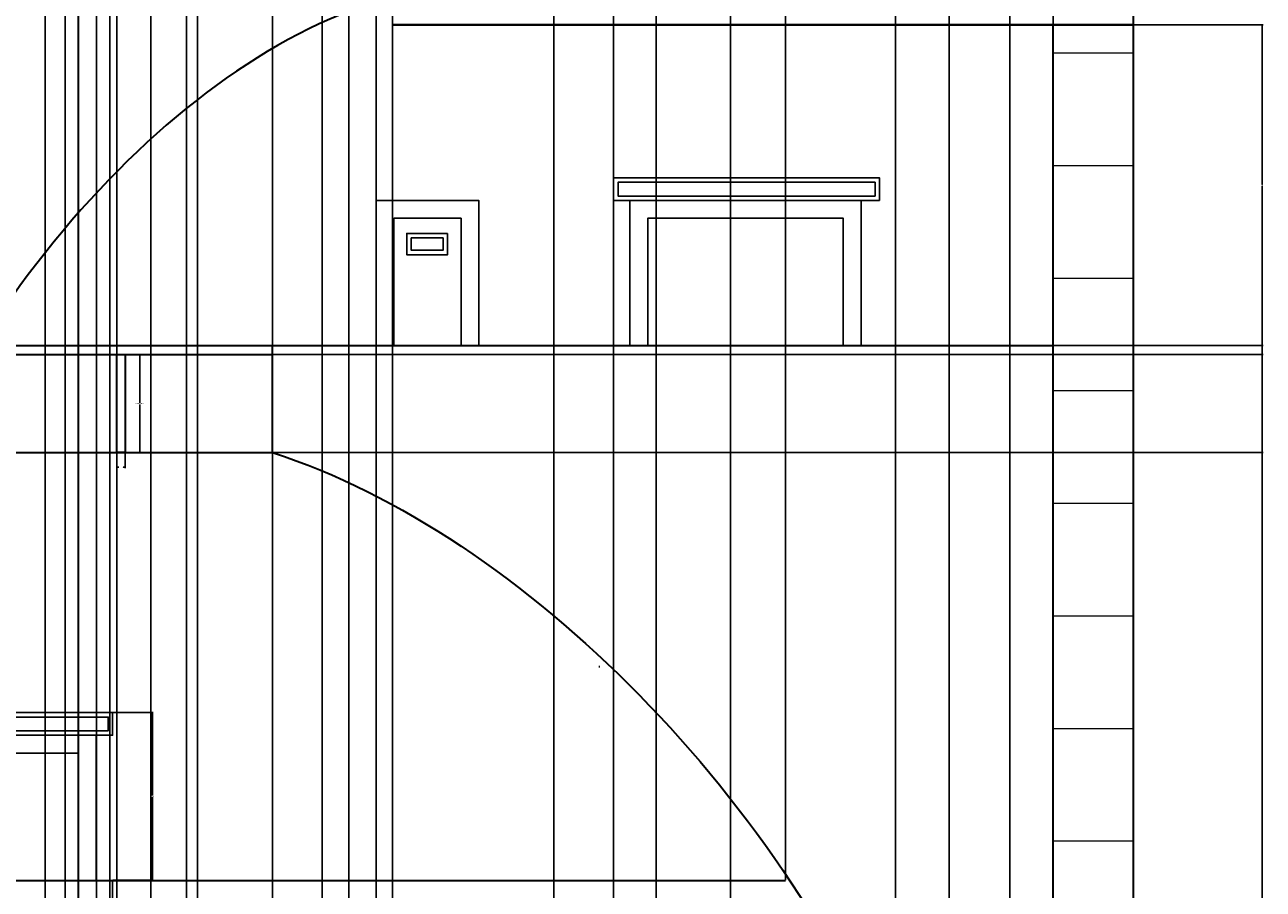
# Model space of a CAD drawing. Units: inches. Extents: x -19 to 408, y -26 to 603.
# Tile 6 of 7: x 130 to 408, y 289 to 483. Entities that reach past the tile are written whole.
import ezdxf

# ---------------------------------------------------------------- set-up
doc = ezdxf.new("R2010")
doc.units = ezdxf.units.IN
doc.header["$MEASUREMENT"] = 0
for name, color, linetype, lineweight in [('A-ANNO-DIMS', 2, 'Continuous', 18), ('A-DOOR', 3, 'Continuous', 25), ('A-ELEV', 7, 'Continuous', 35), ('A-GLAZ', 4, 'Continuous', 25), ('A-WALL-PATT', 8, 'Continuous', 13)]:
    doc.layers.add(name, color=color, linetype=linetype, lineweight=lineweight)
doc.styles.get("Standard").update_dxf_attribs({"font": 'arial.ttf'})
doc.dimstyles.get("Standard").update_dxf_attribs({"dimtxt": 0.18, "dimasz": 0.18, "dimexe": 0.18, "dimexo": 0.0625, "dimgap": 0.09, "dimtad": 0, "dimtih": 1, "dimtoh": 1, "dimdec": 4, "dimzin": 0, "dimdsep": 46, "dimtxsty": 'Standard', "dimcen": 0.09, "dimadec": 0, "dimazin": 0, "dimtfac": 1, "dimtdec": 4, "dimtofl": 0, "dimtmove": 0, "dimatfit": 3, "dimfxl": 1, "dimtolj": 1, "dimtzin": 0, "dimarcsym": 0})

# ---------------------------------------------------------------- blocks, each defined once
blk = doc.blocks.new('WIN-1200')
for points in [[(0, 32.56), (59.66, 32.56), (59.66, 37.64), (0, 37.64)], [(1, 33.56), (58.66, 33.56), (58.66, 36.64), (1, 36.64)]]:
    blk.add_lwpolyline(points, close=True)
for points in [[(4.17, 0), (4.17, 32.56), (55.99, 32.56), (55.99, 0)], [(8.17, 0), (8.17, 28.56), (51.99, 28.56), (51.99, 0)]]:
    blk.add_lwpolyline(points)
blk = doc.blocks.new('DOOR-600')
for points in [[(0, 0), (0, 32.56), (23.06, 32.56), (23.06, 0)], [(4, 0), (4, 28.56), (19.06, 28.56), (19.06, 0)]]:
    blk.add_lwpolyline(points)
for points in [[(7.03, 25.16), (16.18, 25.16), (16.18, 20.4), (7.03, 20.4)], [(8.03, 24.16), (15.18, 24.16), (15.18, 21.4), (8.03, 21.4)]]:
    blk.add_lwpolyline(points, close=True)
blk = doc.blocks.new('RAIL-POST')
blk.add_lwpolyline([(0, 22), (1.83, 22), (1.83, 0), (0, 0)], close=True)
blk = doc.blocks.new('*D4')
at = {"layer": 'A-ANNO-DIMS', "color": 0, "lineweight": -2, "transparency": 16777216}
for p, q in [((89.99, 291.08), (89.99, 282.02)), ((149.65, 291.08), (149.65, 282.02)), ((90.17, 282.2), (118.7, 282.2)), ((149.47, 282.2), (120.94, 282.2))]:
    blk.add_line(p, q, dxfattribs=at)
at = {"layer": 'A-ANNO-DIMS', "color": 0, "transparency": 16777216}
for points in [[(90.17, 282.23), (90.17, 282.17), (89.99, 282.2)], [(149.47, 282.23), (149.47, 282.17), (149.65, 282.2)]]:
    blk.add_solid(points, dxfattribs=at)
at = {"layer": 'Defpoints', "color": 0, "transparency": 16777216}
for p in [(89.99, 291.15), (149.65, 291.15), (149.65, 282.2)]:
    blk.add_point(p, dxfattribs=at)
at = {"layer": 'A-ANNO-DIMS', "color": 0, "transparency": 16777216, "insert": (119.82, 282.2), "char_height": 0.18, "attachment_point": 5}
blk.add_mtext('\\A1;WINDOW 60 TYP.', dxfattribs=at)
blk = doc.blocks.new('*D5')
at = {"layer": 'A-ANNO-DIMS', "color": 0, "lineweight": -2, "transparency": 16777216}
for p, q in [((149.71, 328.79), (158.77, 328.79)), ((158.59, 328.61), (158.59, 310.15)), ((158.59, 291.33), (158.59, 309.79)), ((149.71, 291.15), (158.77, 291.15))]:
    blk.add_line(p, q, dxfattribs=at)
at = {"layer": 'A-ANNO-DIMS', "color": 0, "transparency": 16777216}
for points in [[(158.56, 328.61), (158.62, 328.61), (158.59, 328.79)], [(158.56, 291.33), (158.62, 291.33), (158.59, 291.15)]]:
    blk.add_solid(points, dxfattribs=at)
at = {"layer": 'Defpoints', "color": 0, "transparency": 16777216}
for p in [(149.65, 328.79), (158.59, 328.79), (149.65, 291.15)]:
    blk.add_point(p, dxfattribs=at)
at = {"layer": 'A-ANNO-DIMS', "color": 0, "transparency": 16777216, "insert": (158.59, 309.97), "char_height": 0.18, "attachment_point": 5}
blk.add_mtext('\\A1;38 TYP.', dxfattribs=at)
blk = doc.blocks.new('*D8')
at = {"layer": 'A-ANNO-DIMS', "color": 0, "lineweight": -2, "transparency": 16777216}
for p, q in [((152.51, 409.15), (155.92, 409.15)), ((155.74, 408.97), (155.74, 398.33)), ((155.74, 387.33), (155.74, 397.96)), ((152.51, 387.15), (155.92, 387.15))]:
    blk.add_line(p, q, dxfattribs=at)
at = {"layer": 'A-ANNO-DIMS', "color": 0, "transparency": 16777216}
for points in [[(155.71, 408.97), (155.77, 408.97), (155.74, 409.15)], [(155.71, 387.33), (155.77, 387.33), (155.74, 387.15)]]:
    blk.add_solid(points, dxfattribs=at)
at = {"layer": 'Defpoints', "color": 0, "transparency": 16777216}
for p in [(152.44, 409.15), (155.74, 409.15), (152.44, 387.15)]:
    blk.add_point(p, dxfattribs=at)
at = {"layer": 'A-ANNO-DIMS', "color": 0, "transparency": 16777216, "insert": (155.74, 398.15), "char_height": 0.18, "attachment_point": 5}
blk.add_mtext('\\A1;RAIL POST 22 TYP.', dxfattribs=at)
blk = doc.blocks.new('*D9')
at = {"layer": 'A-ANNO-DIMS', "color": 0, "lineweight": -2, "transparency": 16777216}
for p, q in [((150.62, 387.08), (150.62, 383.67)), ((152.44, 387.08), (152.44, 383.67)), ((150.8, 383.85), (151.07, 383.85)), ((152.26, 383.85), (151.99, 383.85))]:
    blk.add_line(p, q, dxfattribs=at)
at = {"layer": 'A-ANNO-DIMS', "color": 0, "transparency": 16777216}
for points in [[(150.8, 383.88), (150.8, 383.82), (150.62, 383.85)], [(152.26, 383.88), (152.26, 383.82), (152.44, 383.85)]]:
    blk.add_solid(points, dxfattribs=at)
at = {"layer": 'Defpoints', "color": 0, "transparency": 16777216}
for p in [(150.62, 387.15), (152.44, 387.15), (152.44, 383.85)]:
    blk.add_point(p, dxfattribs=at)
at = {"layer": 'A-ANNO-DIMS', "color": 0, "transparency": 16777216, "insert": (151.53, 383.85), "char_height": 0.18, "attachment_point": 5}
blk.add_mtext('\\A1;2 TYP.', dxfattribs=at)
blk = doc.blocks.new('*D20')
at = {"layer": 'A-ANNO-DIMS', "color": 0, "lineweight": -2, "transparency": 16777216}
for p, q in [((185.46, 411.15), (-18.88, 411.15)), ((-18.7, 410.97), (-18.7, 351.33)), ((-18.7, 291.33), (-18.7, 350.97)), ((84.02, 291.15), (-18.88, 291.15))]:
    blk.add_line(p, q, dxfattribs=at)
at = {"layer": 'A-ANNO-DIMS', "color": 0, "transparency": 16777216}
for points in [[(-18.73, 410.97), (-18.67, 410.97), (-18.7, 411.15)], [(-18.73, 291.33), (-18.67, 291.33), (-18.7, 291.15)]]:
    blk.add_solid(points, dxfattribs=at)
at = {"layer": 'Defpoints', "color": 0, "transparency": 16777216}
for p in [(-18.7, 411.15), (185.52, 411.15), (84.08, 291.15)]:
    blk.add_point(p, dxfattribs=at)
at = {"layer": 'A-ANNO-DIMS', "color": 0, "transparency": 16777216, "insert": (-18.7, 351.15), "char_height": 0.18, "attachment_point": 5}
blk.add_mtext('\\A1;120', dxfattribs=at)
blk = doc.blocks.new('*D21')
at = {"layer": 'A-ANNO-DIMS', "color": 0, "lineweight": -2, "transparency": 16777216}
for p, q in [((212.37, 551.1), (-18.88, 551.1)), ((-18.7, 550.92), (-18.7, 481.31)), ((-18.7, 411.33), (-18.7, 480.94)), ((185.46, 411.15), (-18.88, 411.15))]:
    blk.add_line(p, q, dxfattribs=at)
at = {"layer": 'A-ANNO-DIMS', "color": 0, "transparency": 16777216}
for points in [[(-18.73, 550.92), (-18.67, 550.92), (-18.7, 551.1)], [(-18.73, 411.33), (-18.67, 411.33), (-18.7, 411.15)]]:
    blk.add_solid(points, dxfattribs=at)
at = {"layer": 'Defpoints', "color": 0, "transparency": 16777216}
for p in [(-18.7, 551.1), (212.43, 551.1), (185.52, 411.15)]:
    blk.add_point(p, dxfattribs=at)
at = {"layer": 'A-ANNO-DIMS', "color": 0, "transparency": 16777216, "insert": (-18.7, 481.13), "char_height": 0.18, "attachment_point": 5}
blk.add_mtext('\\A1;139.96', dxfattribs=at)
blk = doc.blocks.new('*D23')
at = {"layer": 'A-ANNO-DIMS', "color": 0, "lineweight": -2, "transparency": 16777216}
for p, q in [((360.63, 411.15), (407.65, 411.15)), ((407.47, 410.97), (407.47, 267.33)), ((407.47, 123.33), (407.47, 266.97)), ((360.63, 123.15), (407.65, 123.15))]:
    blk.add_line(p, q, dxfattribs=at)
at = {"layer": 'A-ANNO-DIMS', "color": 0, "transparency": 16777216}
for points in [[(407.44, 410.97), (407.5, 410.97), (407.47, 411.15)], [(407.44, 123.33), (407.5, 123.33), (407.47, 123.15)]]:
    blk.add_solid(points, dxfattribs=at)
at = {"layer": 'Defpoints', "color": 0, "transparency": 16777216}
for p in [(360.57, 411.15), (407.47, 411.15), (360.57, 123.15)]:
    blk.add_point(p, dxfattribs=at)
at = {"layer": 'A-ANNO-DIMS', "color": 0, "transparency": 16777216, "insert": (407.47, 267.15), "char_height": 0.18, "attachment_point": 5}
blk.add_mtext('\\A1;288', dxfattribs=at)
blk = doc.blocks.new('*D24')
at = {"layer": 'A-ANNO-DIMS', "color": 0, "lineweight": -2, "transparency": 16777216}
for p, q in [((378.63, 483.15), (407.65, 483.15)), ((407.47, 482.97), (407.47, 447.33)), ((407.47, 411.33), (407.47, 446.97)), ((360.63, 411.15), (407.65, 411.15))]:
    blk.add_line(p, q, dxfattribs=at)
at = {"layer": 'A-ANNO-DIMS', "color": 0, "transparency": 16777216}
for points in [[(407.44, 482.97), (407.5, 482.97), (407.47, 483.15)], [(407.44, 411.33), (407.5, 411.33), (407.47, 411.15)]]:
    blk.add_solid(points, dxfattribs=at)
at = {"layer": 'Defpoints', "color": 0, "transparency": 16777216}
for p in [(378.57, 483.15), (407.47, 483.15), (360.57, 411.15)]:
    blk.add_point(p, dxfattribs=at)
at = {"layer": 'A-ANNO-DIMS', "color": 0, "transparency": 16777216, "insert": (407.47, 447.15), "char_height": 0.18, "attachment_point": 5}
blk.add_mtext('\\A1;72', dxfattribs=at)
blk = doc.blocks.new('*D27')
at = {"layer": 'A-ANNO-DIMS', "color": 0, "lineweight": -2, "transparency": 16777216}
for p, q in [((288.17, 123.21), (288.17, 602.9)), ((288.35, 602.72), (324.05, 602.72)), ((360.39, 602.72), (324.69, 602.72)), ((360.57, 123.21), (360.57, 602.9))]:
    blk.add_line(p, q, dxfattribs=at)
at = {"layer": 'A-ANNO-DIMS', "color": 0, "transparency": 16777216}
for points in [[(288.35, 602.75), (288.35, 602.69), (288.17, 602.72)], [(360.39, 602.75), (360.39, 602.69), (360.57, 602.72)]]:
    blk.add_solid(points, dxfattribs=at)
at = {"layer": 'Defpoints', "color": 0, "transparency": 16777216}
for p in [(360.57, 602.72), (288.17, 123.15), (360.57, 123.15)]:
    blk.add_point(p, dxfattribs=at)
at = {"layer": 'A-ANNO-DIMS', "color": 0, "transparency": 16777216, "insert": (324.37, 602.72), "char_height": 0.18, "attachment_point": 5}
blk.add_mtext('\\A1;72.4', dxfattribs=at)
blk = doc.blocks.new('*D29')
at = {"layer": 'A-ANNO-DIMS', "color": 0, "lineweight": -2, "transparency": 16777216}
for p, q in [((300.56, 291.21), (300.56, 602.9)), ((300.74, 602.72), (330.19, 602.72)), ((360.39, 602.72), (330.94, 602.72)), ((360.57, 300.05), (360.57, 602.9))]:
    blk.add_line(p, q, dxfattribs=at)
at = {"layer": 'A-ANNO-DIMS', "color": 0, "transparency": 16777216}
for points in [[(300.74, 602.75), (300.74, 602.69), (300.56, 602.72)], [(360.39, 602.75), (360.39, 602.69), (360.57, 602.72)]]:
    blk.add_solid(points, dxfattribs=at)
at = {"layer": 'Defpoints', "color": 0, "transparency": 16777216}
for p in [(360.57, 602.72), (360.57, 299.99), (300.56, 291.15)]:
    blk.add_point(p, dxfattribs=at)
at = {"layer": 'A-ANNO-DIMS', "color": 0, "transparency": 16777216, "insert": (330.56, 602.72), "char_height": 0.18, "attachment_point": 5}
blk.add_mtext('\\A1;60.01', dxfattribs=at)
blk = doc.blocks.new('*D30')
at = {"layer": 'A-ANNO-DIMS', "color": 0, "lineweight": -2, "transparency": 16777216}
for p, q in [((360.57, 411.08), (360.57, -25.93)), ((185.52, 387.08), (185.52, -25.93)), ((185.7, -25.75), (272.59, -25.75)), ((360.39, -25.75), (273.5, -25.75))]:
    blk.add_line(p, q, dxfattribs=at)
at = {"layer": 'A-ANNO-DIMS', "color": 0, "transparency": 16777216}
for points in [[(185.7, -25.72), (185.7, -25.78), (185.52, -25.75)], [(360.39, -25.72), (360.39, -25.78), (360.57, -25.75)]]:
    blk.add_solid(points, dxfattribs=at)
at = {"layer": 'Defpoints', "color": 0, "transparency": 16777216}
for p in [(360.57, 411.15), (185.52, 387.15), (360.57, -25.75)]:
    blk.add_point(p, dxfattribs=at)
at = {"layer": 'A-ANNO-DIMS', "color": 0, "transparency": 16777216, "insert": (273.05, -25.75), "char_height": 0.18, "attachment_point": 5}
blk.add_mtext('\\A1;175.05', dxfattribs=at)
blk = doc.blocks.new('*D36')
at = {"layer": 'A-ANNO-DIMS', "color": 0, "lineweight": -2, "transparency": 16777216}
for p, q in [((52.15, 203.77), (52.15, 602.9)), ((52.33, 602.72), (96.69, 602.72)), ((141.84, 602.72), (97.48, 602.72)), ((142.02, 171.21), (142.02, 602.9))]:
    blk.add_line(p, q, dxfattribs=at)
at = {"layer": 'A-ANNO-DIMS', "color": 0, "transparency": 16777216}
for points in [[(52.33, 602.75), (52.33, 602.69), (52.15, 602.72)], [(141.84, 602.75), (141.84, 602.69), (142.02, 602.72)]]:
    blk.add_solid(points, dxfattribs=at)
at = {"layer": 'Defpoints', "color": 0, "transparency": 16777216}
for p in [(142.02, 602.72), (52.15, 203.7), (142.02, 171.15)]:
    blk.add_point(p, dxfattribs=at)
at = {"layer": 'A-ANNO-DIMS', "color": 0, "transparency": 16777216, "insert": (97.09, 602.72), "char_height": 0.18, "attachment_point": 5}
blk.add_mtext('\\A1;89.87', dxfattribs=at)
blk = doc.blocks.new('*D37')
at = {"layer": 'A-ANNO-DIMS', "color": 0, "lineweight": -2, "transparency": 16777216}
for p, q in [((142.02, 171.21), (142.02, 602.9)), ((142.2, 602.72), (174.97, 602.72)), ((208.53, 602.72), (175.76, 602.72)), ((208.71, 171.21), (208.71, 602.9))]:
    blk.add_line(p, q, dxfattribs=at)
at = {"layer": 'A-ANNO-DIMS', "color": 0, "transparency": 16777216}
for points in [[(142.2, 602.75), (142.2, 602.69), (142.02, 602.72)], [(208.53, 602.75), (208.53, 602.69), (208.71, 602.72)]]:
    blk.add_solid(points, dxfattribs=at)
at = {"layer": 'Defpoints', "color": 0, "transparency": 16777216}
for p in [(208.71, 602.72), (142.02, 171.15), (208.71, 171.15)]:
    blk.add_point(p, dxfattribs=at)
at = {"layer": 'A-ANNO-DIMS', "color": 0, "transparency": 16777216, "insert": (175.37, 602.72), "char_height": 0.18, "attachment_point": 5}
blk.add_mtext('\\A1;66.69', dxfattribs=at)
blk = doc.blocks.new('*D38')
at = {"layer": 'A-ANNO-DIMS', "color": 0, "lineweight": -2, "transparency": 16777216}
for p, q in [((208.71, 171.21), (208.71, 602.9)), ((208.89, 602.72), (234.95, 602.72)), ((261.81, 602.72), (235.74, 602.72)), ((261.99, 203.77), (261.99, 602.9))]:
    blk.add_line(p, q, dxfattribs=at)
at = {"layer": 'A-ANNO-DIMS', "color": 0, "transparency": 16777216}
for points in [[(208.89, 602.75), (208.89, 602.69), (208.71, 602.72)], [(261.81, 602.75), (261.81, 602.69), (261.99, 602.72)]]:
    blk.add_solid(points, dxfattribs=at)
at = {"layer": 'Defpoints', "color": 0, "transparency": 16777216}
for p in [(261.99, 602.72), (261.99, 203.7), (208.71, 171.15)]:
    blk.add_point(p, dxfattribs=at)
at = {"layer": 'A-ANNO-DIMS', "color": 0, "transparency": 16777216, "insert": (235.35, 602.72), "char_height": 0.18, "attachment_point": 5}
blk.add_mtext('\\A1;53.28', dxfattribs=at)
blk = doc.blocks.new('*D45')
at = {"layer": 'A-ANNO-DIMS', "color": 0, "lineweight": -2, "transparency": 16777216}
for p, q in [((36.57, 219.21), (36.57, 602.9)), ((36.75, 602.72), (85.2, 602.72)), ((134.3, 602.72), (85.85, 602.72)), ((134.48, 220.21), (134.48, 602.9))]:
    blk.add_line(p, q, dxfattribs=at)
at = {"layer": 'A-ANNO-DIMS', "color": 0, "transparency": 16777216}
for points in [[(36.75, 602.75), (36.75, 602.69), (36.57, 602.72)], [(134.3, 602.75), (134.3, 602.69), (134.48, 602.72)]]:
    blk.add_solid(points, dxfattribs=at)
at = {"layer": 'Defpoints', "color": 0, "transparency": 16777216}
for p in [(134.48, 602.72), (134.48, 220.15), (36.57, 219.15)]:
    blk.add_point(p, dxfattribs=at)
at = {"layer": 'A-ANNO-DIMS', "color": 0, "transparency": 16777216, "insert": (85.52, 602.72), "char_height": 0.18, "attachment_point": 5}
blk.add_mtext('\\A1;97.9', dxfattribs=at)
blk = doc.blocks.new('*D46')
at = {"layer": 'A-ANNO-DIMS', "color": 0, "lineweight": -2, "transparency": 16777216}
for p, q in [((337.23, 171.21), (337.23, 602.9)), ((337.41, 602.72), (348.43, 602.72)), ((360.39, 602.72), (349.36, 602.72)), ((360.57, 173.74), (360.57, 602.9))]:
    blk.add_line(p, q, dxfattribs=at)
at = {"layer": 'A-ANNO-DIMS', "color": 0, "transparency": 16777216}
for points in [[(337.41, 602.75), (337.41, 602.69), (337.23, 602.72)], [(360.39, 602.75), (360.39, 602.69), (360.57, 602.72)]]:
    blk.add_solid(points, dxfattribs=at)
at = {"layer": 'Defpoints', "color": 0, "transparency": 16777216}
for p in [(360.57, 602.72), (360.57, 173.67), (337.23, 171.15)]:
    blk.add_point(p, dxfattribs=at)
at = {"layer": 'A-ANNO-DIMS', "color": 0, "transparency": 16777216, "insert": (348.9, 602.72), "char_height": 0.18, "attachment_point": 5}
blk.add_mtext('\\A1;23.345', dxfattribs=at)
blk = doc.blocks.new('*D55')
at = {"layer": 'A-ANNO-DIMS', "color": 0, "lineweight": -2, "transparency": 16777216}
for p, q in [((146.02, 199.77), (146.02, 602.9)), ((146.2, 602.72), (147.14, 602.72)), ((148.87, 602.72), (147.93, 602.72)), ((149.05, 196.37), (149.05, 602.9))]:
    blk.add_line(p, q, dxfattribs=at)
at = {"layer": 'A-ANNO-DIMS', "color": 0, "transparency": 16777216}
for points in [[(146.2, 602.75), (146.2, 602.69), (146.02, 602.72)], [(148.87, 602.75), (148.87, 602.69), (149.05, 602.72)]]:
    blk.add_solid(points, dxfattribs=at)
at = {"layer": 'Defpoints', "color": 0, "transparency": 16777216}
for p in [(149.05, 602.72), (146.02, 199.7), (149.05, 196.31)]:
    blk.add_point(p, dxfattribs=at)
at = {"layer": 'A-ANNO-DIMS', "color": 0, "transparency": 16777216, "insert": (147.54, 602.72), "char_height": 0.18, "attachment_point": 5}
blk.add_mtext('\\A1;3.029', dxfattribs=at)
blk = doc.blocks.new('*D56')
at = {"layer": 'A-ANNO-DIMS', "color": 0, "lineweight": -2, "transparency": 16777216}
for p, q in [((149.05, 196.37), (149.05, 602.9)), ((149.23, 602.72), (153.3, 602.72)), ((158.02, 602.72), (153.95, 602.72)), ((158.2, 196.37), (158.2, 602.9))]:
    blk.add_line(p, q, dxfattribs=at)
at = {"layer": 'A-ANNO-DIMS', "color": 0, "transparency": 16777216}
for points in [[(149.23, 602.75), (149.23, 602.69), (149.05, 602.72)], [(158.02, 602.75), (158.02, 602.69), (158.2, 602.72)]]:
    blk.add_solid(points, dxfattribs=at)
at = {"layer": 'Defpoints', "color": 0, "transparency": 16777216}
for p in [(158.2, 602.72), (149.05, 196.31), (158.2, 196.31)]:
    blk.add_point(p, dxfattribs=at)
at = {"layer": 'A-ANNO-DIMS', "color": 0, "transparency": 16777216, "insert": (153.63, 602.72), "char_height": 0.18, "attachment_point": 5}
blk.add_mtext('\\A1;9.15', dxfattribs=at)
blk = doc.blocks.new('*D70')
at = {"layer": 'A-ANNO-DIMS', "color": 0, "lineweight": -2, "transparency": 16777216}
for p, q in [((150.62, 387.08), (150.62, -25.93)), ((185.52, 387.08), (185.52, -25.93)), ((150.8, -25.75), (167.6, -25.75)), ((185.34, -25.75), (168.53, -25.75))]:
    blk.add_line(p, q, dxfattribs=at)
at = {"layer": 'A-ANNO-DIMS', "color": 0, "transparency": 16777216}
for points in [[(150.8, -25.72), (150.8, -25.78), (150.62, -25.75)], [(185.34, -25.72), (185.34, -25.78), (185.52, -25.75)]]:
    blk.add_solid(points, dxfattribs=at)
at = {"layer": 'Defpoints', "color": 0, "transparency": 16777216}
for p in [(150.62, 387.15), (185.52, 387.15), (185.52, -25.75)]:
    blk.add_point(p, dxfattribs=at)
at = {"layer": 'A-ANNO-DIMS', "color": 0, "transparency": 16777216, "insert": (168.07, -25.75), "char_height": 0.18, "attachment_point": 5}
blk.add_mtext('\\A1;34.906', dxfattribs=at)
blk = doc.blocks.new('*D71')
at = {"layer": 'A-ANNO-DIMS', "color": 0, "lineweight": -2, "transparency": 16777216}
for p, q in [((185.58, 409.15), (407.65, 409.15)), ((407.47, 408.97), (407.47, 398.33)), ((407.47, 387.33), (407.47, 397.97)), ((185.58, 387.15), (407.65, 387.15))]:
    blk.add_line(p, q, dxfattribs=at)
at = {"layer": 'A-ANNO-DIMS', "color": 0, "transparency": 16777216}
for points in [[(407.44, 408.97), (407.5, 408.97), (407.47, 409.15)], [(407.44, 387.33), (407.5, 387.33), (407.47, 387.15)]]:
    blk.add_solid(points, dxfattribs=at)
at = {"layer": 'Defpoints', "color": 0, "transparency": 16777216}
for p in [(185.52, 409.15), (407.47, 409.15), (185.52, 387.15)]:
    blk.add_point(p, dxfattribs=at)
at = {"layer": 'A-ANNO-DIMS', "color": 0, "transparency": 16777216, "insert": (407.47, 398.15), "char_height": 0.18, "attachment_point": 5}
blk.add_mtext('\\A1;22', dxfattribs=at)
blk = doc.blocks.new('*D72')
at = {"layer": 'A-ANNO-DIMS', "color": 0, "lineweight": -2, "transparency": 16777216}
for p, q in [((185.58, 411.15), (407.65, 411.15)), ((185.58, 409.15), (407.65, 409.15)), ((407.47, 410.97), (407.47, 410.33)), ((407.47, 409.33), (407.47, 409.97))]:
    blk.add_line(p, q, dxfattribs=at)
at = {"layer": 'A-ANNO-DIMS', "color": 0, "transparency": 16777216}
for points in [[(407.44, 410.97), (407.5, 410.97), (407.47, 411.15)], [(407.44, 409.33), (407.5, 409.33), (407.47, 409.15)]]:
    blk.add_solid(points, dxfattribs=at)
at = {"layer": 'Defpoints', "color": 0, "transparency": 16777216}
for p in [(185.52, 411.15), (407.47, 411.15), (185.52, 409.15)]:
    blk.add_point(p, dxfattribs=at)
at = {"layer": 'A-ANNO-DIMS', "color": 0, "transparency": 16777216, "insert": (407.47, 410.15), "char_height": 0.18, "attachment_point": 5}
blk.add_mtext('\\A1;2', dxfattribs=at)
blk = doc.blocks.new('*D73')
at = {"layer": 'A-ANNO-DIMS', "color": 0, "lineweight": -2, "transparency": 16777216}
for p, q in [((185.52, 411.08), (185.52, -25.93)), ((208.71, 411.08), (208.71, -25.93)), ((185.7, -25.75), (196.72, -25.75)), ((208.53, -25.75), (197.51, -25.75))]:
    blk.add_line(p, q, dxfattribs=at)
at = {"layer": 'A-ANNO-DIMS', "color": 0, "transparency": 16777216}
for points in [[(185.7, -25.72), (185.7, -25.78), (185.52, -25.75)], [(208.53, -25.72), (208.53, -25.78), (208.71, -25.75)]]:
    blk.add_solid(points, dxfattribs=at)
at = {"layer": 'Defpoints', "color": 0, "transparency": 16777216}
for p in [(185.52, 411.15), (208.71, 411.15), (208.71, -25.75)]:
    blk.add_point(p, dxfattribs=at)
at = {"layer": 'A-ANNO-DIMS', "color": 0, "transparency": 16777216, "insert": (197.12, -25.75), "char_height": 0.18, "attachment_point": 5}
blk.add_mtext('\\A1;23.19', dxfattribs=at)
blk = doc.blocks.new('*D74')
at = {"layer": 'A-ANNO-DIMS', "color": 0, "lineweight": -2, "transparency": 16777216}
for p, q in [((208.71, 411.21), (208.71, 602.9)), ((208.89, 602.72), (234.95, 602.72)), ((261.81, 602.72), (235.74, 602.72)), ((261.99, 443.77), (261.99, 602.9))]:
    blk.add_line(p, q, dxfattribs=at)
at = {"layer": 'A-ANNO-DIMS', "color": 0, "transparency": 16777216}
for points in [[(208.89, 602.75), (208.89, 602.69), (208.71, 602.72)], [(261.81, 602.75), (261.81, 602.69), (261.99, 602.72)]]:
    blk.add_solid(points, dxfattribs=at)
at = {"layer": 'Defpoints', "color": 0, "transparency": 16777216}
for p in [(261.99, 602.72), (261.99, 443.7), (208.71, 411.15)]:
    blk.add_point(p, dxfattribs=at)
at = {"layer": 'A-ANNO-DIMS', "color": 0, "transparency": 16777216, "insert": (235.35, 602.72), "char_height": 0.18, "attachment_point": 5}
blk.add_mtext('\\A1;53.28', dxfattribs=at)
blk = doc.blocks.new('*D75')
at = {"layer": 'A-ANNO-DIMS', "color": 0, "lineweight": -2, "transparency": 16777216}
for p, q in [((212.43, 507.08), (212.43, -25.93)), ((248.57, 507.08), (248.57, -25.93)), ((212.61, -25.75), (230.11, -25.75)), ((248.39, -25.75), (230.89, -25.75))]:
    blk.add_line(p, q, dxfattribs=at)
at = {"layer": 'A-ANNO-DIMS', "color": 0, "transparency": 16777216}
for points in [[(212.61, -25.72), (212.61, -25.78), (212.43, -25.75)], [(248.39, -25.72), (248.39, -25.78), (248.57, -25.75)]]:
    blk.add_solid(points, dxfattribs=at)
at = {"layer": 'Defpoints', "color": 0, "transparency": 16777216}
for p in [(212.43, 507.15), (248.57, 507.15), (248.57, -25.75)]:
    blk.add_point(p, dxfattribs=at)
at = {"layer": 'A-ANNO-DIMS', "color": 0, "transparency": 16777216, "insert": (230.5, -25.75), "char_height": 0.18, "attachment_point": 5}
blk.add_mtext('\\A1;36.14', dxfattribs=at)
blk = doc.blocks.new('*D76')
at = {"layer": 'A-ANNO-DIMS', "color": 0, "lineweight": -2, "transparency": 16777216}
for p, q in [((248.57, 507.08), (248.57, -25.93)), ((271.51, 507.08), (271.51, -25.93)), ((248.75, -25.75), (259.58, -25.75)), ((271.33, -25.75), (260.51, -25.75))]:
    blk.add_line(p, q, dxfattribs=at)
at = {"layer": 'A-ANNO-DIMS', "color": 0, "transparency": 16777216}
for points in [[(248.75, -25.72), (248.75, -25.78), (248.57, -25.75)], [(271.33, -25.72), (271.33, -25.78), (271.51, -25.75)]]:
    blk.add_solid(points, dxfattribs=at)
at = {"layer": 'Defpoints', "color": 0, "transparency": 16777216}
for p in [(248.57, 507.15), (271.51, 507.15), (271.51, -25.75)]:
    blk.add_point(p, dxfattribs=at)
at = {"layer": 'A-ANNO-DIMS', "color": 0, "transparency": 16777216, "insert": (260.04, -25.75), "char_height": 0.18, "attachment_point": 5}
blk.add_mtext('\\A1;22.944', dxfattribs=at)
blk = doc.blocks.new('*D77')
at = {"layer": 'A-ANNO-DIMS', "color": 0, "lineweight": -2, "transparency": 16777216}
for p, q in [((271.51, 507.08), (271.51, -25.93)), ((325.24, 507.08), (325.24, -25.93)), ((271.69, -25.75), (297.98, -25.75)), ((325.06, -25.75), (298.77, -25.75))]:
    blk.add_line(p, q, dxfattribs=at)
at = {"layer": 'A-ANNO-DIMS', "color": 0, "transparency": 16777216}
for points in [[(271.69, -25.72), (271.69, -25.78), (271.51, -25.75)], [(325.06, -25.72), (325.06, -25.78), (325.24, -25.75)]]:
    blk.add_solid(points, dxfattribs=at)
at = {"layer": 'Defpoints', "color": 0, "transparency": 16777216}
for p in [(271.51, 507.15), (325.24, 507.15), (325.24, -25.75)]:
    blk.add_point(p, dxfattribs=at)
at = {"layer": 'A-ANNO-DIMS', "color": 0, "transparency": 16777216, "insert": (298.38, -25.75), "char_height": 0.18, "attachment_point": 5}
blk.add_mtext('\\A1;53.72', dxfattribs=at)
blk = doc.blocks.new('*D78')
at = {"layer": 'A-ANNO-DIMS', "color": 0, "lineweight": -2, "transparency": 16777216}
for p, q in [((325.24, 507.08), (325.24, -25.93)), ((350.82, 507.08), (350.82, -25.93)), ((325.42, -25.75), (337.56, -25.75)), ((350.64, -25.75), (338.49, -25.75))]:
    blk.add_line(p, q, dxfattribs=at)
at = {"layer": 'A-ANNO-DIMS', "color": 0, "transparency": 16777216}
for points in [[(325.42, -25.72), (325.42, -25.78), (325.24, -25.75)], [(350.64, -25.72), (350.64, -25.78), (350.82, -25.75)]]:
    blk.add_solid(points, dxfattribs=at)
at = {"layer": 'Defpoints', "color": 0, "transparency": 16777216}
for p in [(325.24, 507.15), (350.82, 507.15), (350.82, -25.75)]:
    blk.add_point(p, dxfattribs=at)
at = {"layer": 'A-ANNO-DIMS', "color": 0, "transparency": 16777216, "insert": (338.03, -25.75), "char_height": 0.18, "attachment_point": 5}
blk.add_mtext('\\A1;25.584', dxfattribs=at)
blk = doc.blocks.new('*D83')
at = {"layer": 'A-ANNO-DIMS', "color": 0, "lineweight": -2, "transparency": 16777216}
for p, q in [((141.92, 491.44), (141.92, -25.93)), ((166.23, 491.44), (166.23, -25.93)), ((142.1, -25.75), (153.69, -25.75)), ((166.05, -25.75), (154.45, -25.75))]:
    blk.add_line(p, q, dxfattribs=at)
at = {"layer": 'A-ANNO-DIMS', "color": 0, "transparency": 16777216}
for points in [[(142.1, -25.72), (142.1, -25.78), (141.92, -25.75)], [(166.05, -25.72), (166.05, -25.78), (166.23, -25.75)]]:
    blk.add_solid(points, dxfattribs=at)
at = {"layer": 'Defpoints', "color": 0, "transparency": 16777216}
for p in [(141.92, 491.5), (166.23, 491.5), (166.23, -25.75)]:
    blk.add_point(p, dxfattribs=at)
at = {"layer": 'A-ANNO-DIMS', "color": 0, "transparency": 16777216, "insert": (154.07, -25.75), "char_height": 0.18, "attachment_point": 5}
blk.add_mtext('\\A1;24.31', dxfattribs=at)
blk = doc.blocks.new('*D84')
at = {"layer": 'A-ANNO-DIMS', "color": 0, "lineweight": -2, "transparency": 16777216}
for p, q in [((138.97, 531.28), (138.97, -25.93)), ((168.64, 531.28), (168.64, -25.93)), ((139.15, -25.75), (153.41, -25.75)), ((168.46, -25.75), (154.2, -25.75))]:
    blk.add_line(p, q, dxfattribs=at)
at = {"layer": 'A-ANNO-DIMS', "color": 0, "transparency": 16777216}
for points in [[(139.15, -25.72), (139.15, -25.78), (138.97, -25.75)], [(168.46, -25.72), (168.46, -25.78), (168.64, -25.75)]]:
    blk.add_solid(points, dxfattribs=at)
at = {"layer": 'Defpoints', "color": 0, "transparency": 16777216}
for p in [(138.97, 531.34), (168.64, 531.34), (168.64, -25.75)]:
    blk.add_point(p, dxfattribs=at)
at = {"layer": 'A-ANNO-DIMS', "color": 0, "transparency": 16777216, "insert": (153.81, -25.75), "char_height": 0.18, "attachment_point": 5}
blk.add_mtext('\\A1;29.67', dxfattribs=at)
blk = doc.blocks.new('*D95')
at = {"layer": 'A-ANNO-DIMS', "color": 0, "lineweight": -2, "transparency": 16777216}
for p, q in [((150.57, 85.97), (150.57, 602.9)), ((150.75, 602.72), (173.31, 602.72)), ((196.49, 602.72), (173.93, 602.72)), ((196.67, 85.97), (196.67, 602.9))]:
    blk.add_line(p, q, dxfattribs=at)
at = {"layer": 'A-ANNO-DIMS', "color": 0, "transparency": 16777216}
for points in [[(150.75, 602.75), (150.75, 602.69), (150.57, 602.72)], [(196.49, 602.75), (196.49, 602.69), (196.67, 602.72)]]:
    blk.add_solid(points, dxfattribs=at)
at = {"layer": 'Defpoints', "color": 0, "transparency": 16777216}
for p in [(196.67, 602.72), (150.57, 85.9), (196.67, 85.9)]:
    blk.add_point(p, dxfattribs=at)
at = {"layer": 'A-ANNO-DIMS', "color": 0, "transparency": 16777216, "insert": (173.62, 602.72), "char_height": 0.18, "attachment_point": 5}
blk.add_mtext('\\A1;46.1', dxfattribs=at)
blk = doc.blocks.new('*D96')
at = {"layer": 'A-ANNO-DIMS', "color": 0, "lineweight": -2, "transparency": 16777216}
for p, q in [((196.67, 85.97), (196.67, 602.9)), ((196.85, 602.72), (199.31, 602.72)), ((202.41, 602.72), (199.96, 602.72)), ((202.59, 85.97), (202.59, 602.9))]:
    blk.add_line(p, q, dxfattribs=at)
at = {"layer": 'A-ANNO-DIMS', "color": 0, "transparency": 16777216}
for points in [[(196.85, 602.75), (196.85, 602.69), (196.67, 602.72)], [(202.41, 602.75), (202.41, 602.69), (202.59, 602.72)]]:
    blk.add_solid(points, dxfattribs=at)
at = {"layer": 'Defpoints', "color": 0, "transparency": 16777216}
for p in [(202.59, 602.72), (196.67, 85.9), (202.59, 85.9)]:
    blk.add_point(p, dxfattribs=at)
at = {"layer": 'A-ANNO-DIMS', "color": 0, "transparency": 16777216, "insert": (199.63, 602.72), "char_height": 0.18, "attachment_point": 5}
blk.add_mtext('\\A1;5.92', dxfattribs=at)
blk = doc.blocks.new('*D105')
at = {"layer": 'A-ANNO-DIMS', "color": 0, "lineweight": -2, "transparency": 16777216}
for p, q in [((120.05, 411.21), (120.05, 602.9)), ((120.23, 602.72), (152.39, 602.72)), ((185.34, 602.72), (153.18, 602.72)), ((185.52, 411.21), (185.52, 602.9))]:
    blk.add_line(p, q, dxfattribs=at)
at = {"layer": 'A-ANNO-DIMS', "color": 0, "transparency": 16777216}
for points in [[(120.23, 602.75), (120.23, 602.69), (120.05, 602.72)], [(185.34, 602.75), (185.34, 602.69), (185.52, 602.72)]]:
    blk.add_solid(points, dxfattribs=at)
at = {"layer": 'Defpoints', "color": 0, "transparency": 16777216}
for p in [(120.05, 602.72), (120.05, 411.15), (185.52, 411.15)]:
    blk.add_point(p, dxfattribs=at)
at = {"layer": 'A-ANNO-DIMS', "color": 0, "transparency": 16777216, "insert": (152.79, 602.72), "char_height": 0.18, "attachment_point": 5}
blk.add_mtext('\\A1;65.47', dxfattribs=at)
blk = doc.blocks.new('*D106')
at = {"layer": 'A-ANNO-DIMS', "color": 0, "lineweight": -2, "transparency": 16777216}
for p, q in [((106.54, 387.08), (106.54, -25.93)), ((185.52, 387.08), (185.52, -25.93)), ((106.72, -25.75), (145.64, -25.75)), ((185.34, -25.75), (146.43, -25.75))]:
    blk.add_line(p, q, dxfattribs=at)
at = {"layer": 'A-ANNO-DIMS', "color": 0, "transparency": 16777216}
for points in [[(106.72, -25.72), (106.72, -25.78), (106.54, -25.75)], [(185.34, -25.72), (185.34, -25.78), (185.52, -25.75)]]:
    blk.add_solid(points, dxfattribs=at)
at = {"layer": 'Defpoints', "color": 0, "transparency": 16777216}
for p in [(106.54, 387.15), (185.52, 387.15), (106.54, -25.75)]:
    blk.add_point(p, dxfattribs=at)
at = {"layer": 'A-ANNO-DIMS', "color": 0, "transparency": 16777216, "insert": (146.03, -25.75), "char_height": 0.18, "attachment_point": 5}
blk.add_mtext('\\A1;78.98', dxfattribs=at)

msp = doc.modelspace()

# ---------------------------------------------------------------- linework, layer by layer
at = {"layer": 'A-ELEV'}
for p, q in [((378.5712, 483.1472), (378.5712, 531.1472)), ((378.5712, 483.1472), (212.4303, 483.1472)), ((212.4303, 483.1472), (378.5712, 483.1472)), ((360.5712, 123.1472), (360.5712, 483.1472)), ((378.5712, 123.1472), (378.5712, 483.1472)), ((120.0489, 411.1472), (360.5712, 411.1472)), ((185.5212, 387.1472), (185.5212, 411.1472)), ((118.7171, 409.1472), (185.5212, 409.1472)), ((106.5444, 387.1472), (185.5212, 387.1472)), ((258.6434, 339.1472), (258.935, 339.1472)), ((84.0785, 291.1472), (300.5581, 291.1472))]:
    msp.add_line(p, q, dxfattribs=at)
msp.add_ellipse((188.4962, 355.8525), major_axis=(71.2607, 129.8447), ratio=0.58959924, start_param=6.80188927, end_param=9.63162337, dxfattribs=at)
at = {"layer": 'A-ELEV', "extrusion": (0, 0, -1)}
msp.add_ellipse((217.8094, 257.6617), major_axis=(99.7631, -123.1178), ratio=0.55109141, start_param=3.84421936, end_param=6.63412911, dxfattribs=at)
at = {"layer": 'A-WALL-PATT'}
for p, q in [((360.5712, 476.8314), (378.5712, 476.8314)), ((360.5712, 451.5683), (378.5712, 451.5683)), ((360.5712, 426.3051), (378.5712, 426.3051)), ((360.5712, 401.042), (378.5712, 401.042)), ((360.5712, 375.7788), (378.5712, 375.7788)), ((360.5712, 350.5157), (378.5712, 350.5157)), ((360.5712, 325.2525), (378.5712, 325.2525)), ((360.5712, 299.9893), (378.5712, 299.9893))]:
    msp.add_line(p, q, dxfattribs=at)

# ---------------------------------------------------------------- block references
at = {"layer": 'A-DOOR', "extrusion": (0, 0, -1), "zscale": -1}
msp.add_blockref('DOOR-600', (-231.7733, 411.147), dxfattribs=at)
at = {"layer": 'A-ELEV'}
msp.add_blockref('RAIL-POST', (150.615, 387.147), dxfattribs=at)
at = {"layer": 'A-GLAZ', "extrusion": (0, 0, -1), "zscale": -1}
msp.add_blockref('WIN-1200', (-321.6443, 411.147), dxfattribs=at)
at = {"layer": 'A-GLAZ'}
msp.add_blockref('WIN-1200', (89.9903, 291.147), dxfattribs=at)

# ---------------------------------------------------------------- dimensions: what is measured, and where the dimension line sits
at = {"layer": 'A-ANNO-DIMS'}
for base, p1, p2, override, picture, middle in [((134.4772, 602.7184), (36.5712, 219.1472), (134.4772, 220.1467), {"dimdec": 1, "dimlfac": 1, "dimrnd": 0, "dimzin": 0, "dimdsep": 46, "dimlunit": 2}, '*D45', (85.5242, 602.7184)), ((142.0243, 602.7184), (52.1528, 203.704), (142.0243, 171.1472), {"dimdec": 2, "dimlfac": 1, "dimrnd": 0, "dimzin": 0, "dimdsep": 46, "dimlunit": 2}, '*D36', (97.0885, 602.7184)), ((120.0489, 602.7184), (185.5212, 411.1472), (120.0489, 411.1472), {"dimdec": 2, "dimlfac": 1, "dimrnd": 0, "dimzin": 0, "dimdsep": 46, "dimlunit": 2}, '*D105', (152.7851, 602.7184)), ((208.70929, 602.71845), (142.02426, 171.14723), (208.70929, 171.14723), {"dimdec": 2, "dimlfac": 1, "dimrnd": 0, "dimzin": 0, "dimdsep": 46, "dimlunit": 2}, '*D37', (175.36677, 602.71845)), ((149.0532, 602.7184), (146.0243, 199.704), (149.0532, 196.3059), {"dimdec": 3, "dimlfac": 1, "dimrnd": 0, "dimzin": 0, "dimdsep": 46, "dimlunit": 2}, '*D55', (147.5387, 602.7184)), ((158.2025, 602.7184), (149.0532, 196.3059), (158.2025, 196.3059), {"dimdec": 2, "dimlfac": 1, "dimrnd": 0, "dimzin": 0, "dimdsep": 46, "dimlunit": 2}, '*D56', (153.6278, 602.7184)), ((196.6731, 602.7184), (150.5712, 85.9033), (196.6731, 85.9033), {"dimdec": 1, "dimlfac": 1, "dimrnd": 0, "dimzin": 0, "dimdsep": 46, "dimlunit": 2}, '*D95', (173.6222, 602.7184)), ((202.5934, 602.7184), (196.6731, 85.9033), (202.5934, 85.9033), {"dimdec": 2, "dimlfac": 1, "dimrnd": 0, "dimzin": 0, "dimdsep": 46, "dimlunit": 2}, '*D96', (199.6333, 602.7184)), ((261.9882, 602.7184), (208.7093, 171.1472), (261.9882, 203.704), {"dimdec": 2, "dimlfac": 1, "dimrnd": 0, "dimzin": 0, "dimdsep": 46, "dimlunit": 2}, '*D38', (235.3487, 602.7184)), ((261.9882, 602.7184), (208.7093, 411.1472), (261.9882, 443.704), {"dimdec": 2, "dimlfac": 1, "dimrnd": 0, "dimzin": 0, "dimdsep": 46, "dimlunit": 2}, '*D74', (235.3487, 602.7184)), ((360.5712, 602.7184), (288.1664, 123.1472), (360.5712, 123.1472), {"dimdec": 1, "dimlfac": 1, "dimrnd": 0, "dimzin": 0, "dimdsep": 46, "dimlunit": 2}, '*D27', (324.3688, 602.7184)), ((360.5712, 602.7184), (300.5581, 291.1472), (360.5712, 299.9893), {"dimdec": 2, "dimlfac": 1, "dimrnd": 0, "dimzin": 0, "dimdsep": 46, "dimlunit": 2}, '*D29', (330.5647, 602.7184)), ((360.5712, 602.7184), (337.2261, 171.1472), (360.5712, 173.6736), {"dimdec": 3, "dimlfac": 1, "dimrnd": 0, "dimzin": 0, "dimdsep": 46, "dimlunit": 2}, '*D46', (348.8986, 602.7184)), ((168.6421, -25.7528), (138.9724, 531.3421), (168.6421, 531.3421), {"dimdec": 2, "dimlfac": 1, "dimrnd": 0, "dimzin": 0, "dimdsep": 46, "dimlunit": 2}, '*D84', (153.8072, -25.7528)), ((248.5703, -25.7528), (212.4303, 507.1472), (248.5703, 507.1472), {"dimdec": 2, "dimlfac": 1, "dimrnd": 0, "dimzin": 0, "dimdsep": 46, "dimlunit": 2}, '*D75', (230.5003, -25.7528)), ((271.514, -25.7528), (248.5703, 507.1472), (271.514, 507.1472), {"dimdec": 3, "dimlfac": 1, "dimrnd": 0, "dimzin": 0, "dimdsep": 46, "dimlunit": 2}, '*D76', (260.0422, -25.7528)), ((325.2366, -25.7528), (271.514, 507.1472), (325.2366, 507.1472), {"dimdec": 2, "dimlfac": 1, "dimrnd": 0, "dimzin": 0, "dimdsep": 46, "dimlunit": 2}, '*D77', (298.3753, -25.7528)), ((350.8209, -25.7528), (325.2366, 507.1472), (350.8209, 507.1472), {"dimdec": 3, "dimlfac": 1, "dimrnd": 0, "dimzin": 0, "dimdsep": 46, "dimlunit": 2}, '*D78', (338.0288, -25.7528)), ((166.228, -25.7528), (141.9163, 491.5037), (166.228, 491.5037), {"dimdec": 2, "dimlfac": 1, "dimrnd": 0, "dimzin": 0, "dimdsep": 46, "dimlunit": 2}, '*D83', (154.0722, -25.7528)), ((360.5712, -25.7528), (185.5212, 387.1472), (360.5712, 411.1472), {"dimdec": 2, "dimlfac": 1, "dimrnd": 0, "dimzin": 0, "dimdsep": 46, "dimlunit": 2}, '*D30', (273.0462, -25.7528)), ((208.7093, -25.7528), (185.5212, 411.1472), (208.7093, 411.1472), {"dimdec": 2, "dimlfac": 1, "dimrnd": 0, "dimzin": 0, "dimdsep": 46, "dimlunit": 2}, '*D73', (197.1153, -25.7528)), ((106.5444, -25.7528), (185.5212, 387.1472), (106.5444, 387.1472), {"dimdec": 2, "dimlfac": 1, "dimrnd": 0, "dimzin": 0, "dimdsep": 46, "dimlunit": 2}, '*D106', (146.0328, -25.7528)), ((185.5212, -25.7528), (150.6152, 387.1472), (185.5212, 387.1472), {"dimdec": 3, "dimlfac": 1, "dimrnd": 0, "dimzin": 0, "dimdsep": 46, "dimlunit": 2}, '*D70', (168.0682, -25.7528))]:
    dim = msp.add_linear_dim(base=base, p1=p1, p2=p2, dimstyle='Standard', override=override, dxfattribs=at)
    dim.commit()
    dim.dimension.update_dxf_attribs({"geometry": picture, "text_midpoint": middle})
for base, p1, p2, override, picture, middle in [((-18.698, 551.1043), (185.5212, 411.1472), (212.4303, 551.1043), {"dimdec": 2, "dimlfac": 1, "dimrnd": 0, "dimzin": 0, "dimdsep": 46, "dimlunit": 2}, '*D21', (-18.698, 481.1258)), ((407.4712, 483.1472), (360.5712, 411.1472), (378.5712, 483.1472), {"dimdec": 0, "dimlfac": 1, "dimrnd": 0, "dimzin": 0, "dimdsep": 46, "dimlunit": 2}, '*D24', (407.4712, 447.1472)), ((-18.698, 411.1472), (84.0785, 291.1472), (185.5212, 411.1472), {"dimdec": 0, "dimlfac": 1, "dimrnd": 0, "dimzin": 0, "dimdsep": 46, "dimlunit": 2}, '*D20', (-18.698, 351.1472)), ((407.4712, 411.1472), (185.5212, 409.1472), (185.5212, 411.1472), {"dimdec": 0, "dimlfac": 1, "dimrnd": 0, "dimzin": 0, "dimdsep": 46, "dimlunit": 2}, '*D72', (407.4712, 410.1472)), ((407.4712, 411.1472), (360.5712, 123.1472), (360.5712, 411.1472), {"dimdec": 0, "dimlfac": 1, "dimrnd": 0, "dimzin": 0, "dimdsep": 46, "dimlunit": 2}, '*D23', (407.4712, 267.1472)), ((407.4712, 409.1472), (185.5212, 387.1472), (185.5212, 409.1472), {"dimdec": 0, "dimlfac": 1, "dimrnd": 0, "dimzin": 0, "dimdsep": 46, "dimlunit": 2}, '*D71', (407.4712, 398.1472))]:
    dim = msp.add_linear_dim(base=base, p1=p1, p2=p2, angle=90, dimstyle='Standard', override=override, dxfattribs=at)
    dim.commit()
    dim.dimension.update_dxf_attribs({"geometry": picture, "text_midpoint": middle})
for base, p1, p2, text, picture, middle in [((155.7428, 409.1472), (152.4428, 387.1472), (152.4428, 409.1472), 'RAIL POST <> TYP.', '*D8', (155.7428, 398.1472)), ((158.5949, 328.7903), (149.6464, 291.1472), (149.6464, 328.7903), '<> TYP.', '*D5', (158.5949, 309.9688))]:
    dim = msp.add_linear_dim(base=base, p1=p1, p2=p2, angle=90, text=text, dimstyle='Standard', override={"dimdec": 0, "dimlfac": 1, "dimrnd": 0, "dimzin": 0, "dimdsep": 46, "dimlunit": 2}, dxfattribs=at)
    dim.commit()
    dim.dimension.update_dxf_attribs({"geometry": picture, "text_midpoint": middle})
for base, p1, p2, text, picture, middle in [((152.4428, 383.8472), (150.6152, 387.1472), (152.4428, 387.1472), '<> TYP.', '*D9', (151.529, 383.8472)), ((149.6464, 282.1988), (89.9901, 291.1472), (149.6464, 291.1472), 'WINDOW <> TYP.', '*D4', (119.8182, 282.1988))]:
    dim = msp.add_linear_dim(base=base, p1=p1, p2=p2, text=text, dimstyle='Standard', override={"dimdec": 0, "dimlfac": 1, "dimrnd": 0, "dimzin": 0, "dimdsep": 46, "dimlunit": 2}, dxfattribs=at)
    dim.commit()
    dim.dimension.update_dxf_attribs({"geometry": picture, "text_midpoint": middle})

doc.saveas('drawing.dxf')
